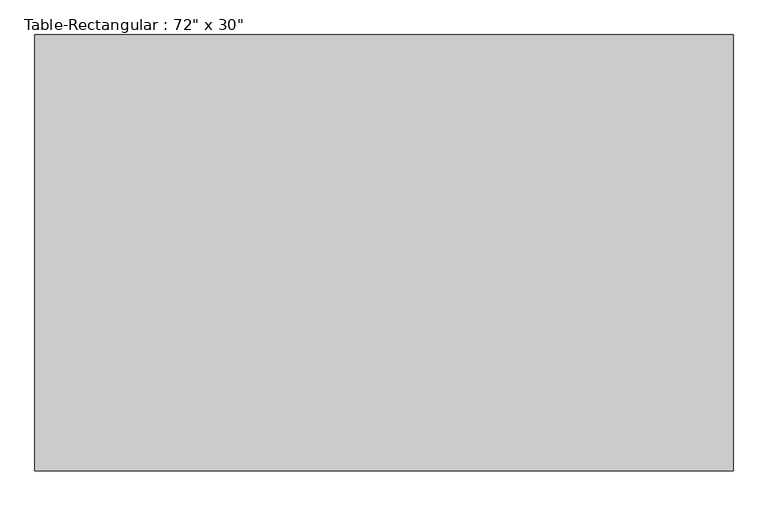
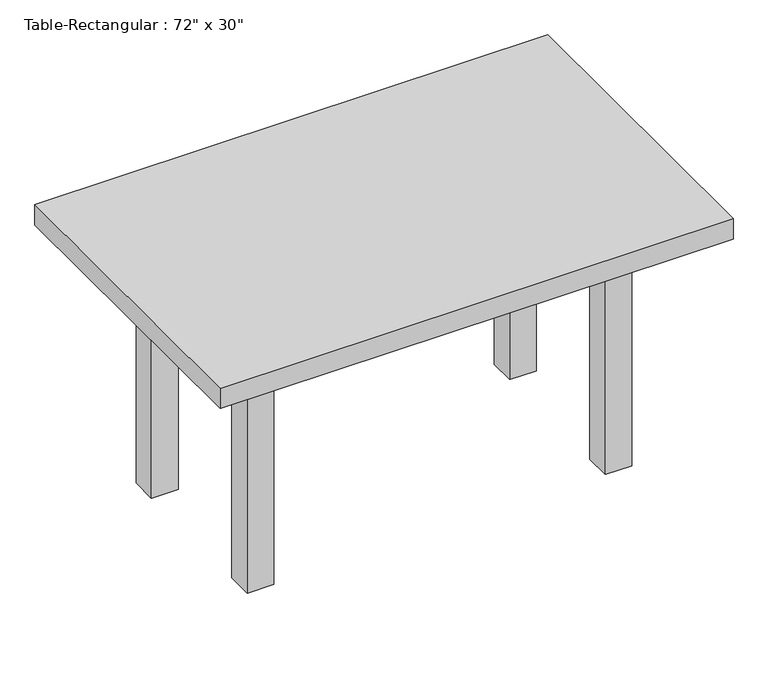
"""IFC4 building model written with IfcOpenShell, lengths in millimetres: furniture geometry."""

from ifc_helpers import new_model, si_unit, frame, origin, origin_with_axes, place, context, project, spatial, polyline, outline, extrude, source, transform, mapped, element, save


def furniture_3f969c1c(model_context):
    return source(origin(), model_context, "Body", "SweptSolid", [
        extrude(outline(polyline([(393.7, 190.5), (393.7, 165.1), (-393.7, 165.1), (-393.7, 190.5), (393.7, 190.5)])), frame((0.0, 0.0, 508.0), z_axis=(0.0, 0.0, 1.0), x_axis=(1.0, 0.0, 0.0)), (0.0, 0.0, 1.0), 101.6),
        extrude(outline(polyline([(393.7, -190.5), (-393.7, -190.5), (-393.7, -165.1), (393.7, -165.1), (393.7, -190.5)])), frame((0.0, 0.0, 508.0), z_axis=(0.0, 0.0, 1.0), x_axis=(1.0, 0.0, 0.0)), (0.0, 0.0, 1.0), 101.6),
        extrude(outline(polyline([(-406.4, -165.1), (-431.8, -165.1), (-431.8, 165.1), (-406.4, 165.1), (-406.4, -165.1)])), frame((0.0, 0.0, 508.0), z_axis=(0.0, 0.0, 1.0), x_axis=(1.0, 0.0, 0.0)), (0.0, 0.0, 1.0), 101.6),
        extrude(outline(polyline([(406.4, -165.1), (406.4, 165.1), (431.8, 165.1), (431.8, -165.1), (406.4, -165.1)])), frame((0.0, 0.0, 508.0), z_axis=(0.0, 0.0, 1.0), x_axis=(1.0, 0.0, 0.0)), (0.0, 0.0, 1.0), 101.6),
        extrude(outline(polyline([(609.6, 381.0), (609.6, -381.0), (-609.6, -381.0), (-609.6, 381.0), (609.6, 381.0)])), frame((0.0, 0.0, 609.6), z_axis=(0.0, 0.0, 1.0), x_axis=(1.0, 0.0, 0.0)), (0.0, 0.0, 1.0), 50.8),
        extrude(outline(polyline([(-393.7, 228.6), (-393.7, 165.1), (-457.2, 165.1), (-457.2, 228.6), (-393.7, 228.6)])), origin_with_axes(), (0.0, 0.0, 1.0), 609.6),
        extrude(outline(polyline([(393.7, 228.6), (457.2, 228.6), (457.2, 165.1), (393.7, 165.1), (393.7, 228.6)])), origin_with_axes(), (0.0, 0.0, 1.0), 609.6),
        extrude(outline(polyline([(-393.7, -228.6), (-457.2, -228.6), (-457.2, -165.1), (-393.7, -165.1), (-393.7, -228.6)])), origin_with_axes(), (0.0, 0.0, 1.0), 609.6),
        extrude(outline(polyline([(393.7, -228.6), (393.7, -165.1), (457.2, -165.1), (457.2, -228.6), (393.7, -228.6)])), origin_with_axes(), (0.0, 0.0, 1.0), 609.6),
    ])


if __name__ == "__main__":
    model = new_model("IFC4")
    model_context = context("Model", 3, world=origin())
    ifc_project = project(units=[si_unit("LENGTHUNIT", "METRE", prefix="MILLI")], contexts=[model_context])
    site = spatial("IfcSite", under=ifc_project)
    building = spatial("IfcBuilding", under=site)
    placement = place(None, origin())
    furniture_shape = furniture_3f969c1c(model_context)
    element("IfcFurniture", 1, ObjectType="Table-Rectangular : 72\" x 30\"", at=placement, inside=building, context=model_context, shape_type="MappedRepresentation", body=[
        mapped(furniture_shape, transform((0.0, 0.0, 0.0), x_axis=(1.0, 0.0, 0.0), y_axis=(0.0, 1.0, 0.0), z_axis=(0.0, 0.0, 1.0))),
    ])
    save(model, "model.ifc")

# Revit data of these elements
# Type "Table-Rectangular : 72\" x 30\""
#   Assembly Code = "E2020200"
#   Height = 2' - 2"
#   Length = 4' - 0"
#   Width = 2' - 6"
#   Base Material = Birch
#   Top Material = Birch
#   Default Elevation = 0
# Element 1 (IfcFurniture, "Table-Rectangular : 72\" x 30\"")
#   Materials on its faces: "Birch"
# Materials
#   "Birch": class "Wood", colour RGB 210 159 95, transparency 0, Description = "Betula Alleghaniensis", Cost = 0
